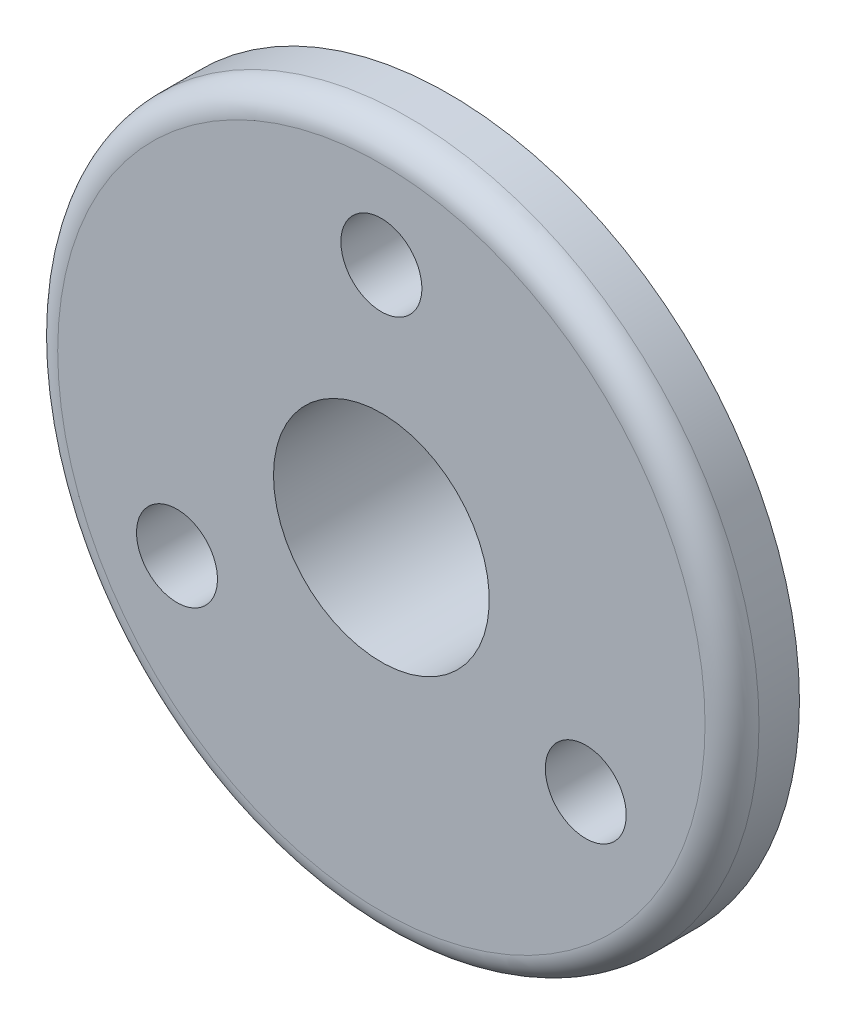
SolidWorks part; units mm, degrees
material "Plain Carbon Steel"
ref_plane "Front Plane" through (0, 0, 0) normal (0, 0, 1) x (1, 0, 0)
ref_plane "Top Plane" through (0, 0, 0) normal (0, 1, 0) x (1, 0, 0)
ref_plane "Right Plane" through (0, 0, 0) normal (1, 0, 0) x (0, 0, -1)
sketch "Flange Profile" plane through (0, 0, 0) normal (0, 0, 1) x (1, 0, 0)
  circle A0 centre (0, 0) radius 26
  dimension "D1" = 52
extrude "Flange Ø52" add sketch "Flange Profile" against normal blind 5
sketch "Hub Profile" plane through (0, 0, -5) normal (0, 0, -1) x (-1, 0, 0)
  circle A0 centre (0, 0) radius 12.5
  dimension "D1" = 25
extrude "Hub Ø25" add sketch "Hub Profile" along normal blind 7
sketch "Bore Profile" plane through (0, 0, -12) normal (0, 0, -1) x (-1, 0, 0)
  circle A0 centre (0, 0) radius 8
  dimension "D1" = 16
extrude "Bore Ø16" cut sketch "Bore Profile" against normal through all both
sketch "Bolt Hole Profile" plane through (0, 0, -5) normal (0, 0, -1) x (-1, 0, 0)
  line L0 (0, -28.5848) -> (0, 27.6798) construction
  line L1 (-29.4899, 0) -> (31.3754, 0) construction
  circle A0 centre (0, 17.5) radius 3
  circle A1 centre (0, 0) radius 17.5 construction
  circle A2 centre (15.1554, -8.75) radius 3
  circle A3 centre (-15.1554, -8.75) radius 3
  point P11 (0, 0)
  dimension "D1" = 6
  dimension "D2" = 35
  dimension "D3" = 3
extrude "Bolt Holes 3xØ6 PCD35" cut sketch "Bolt Hole Profile" against normal through all both
fillet "Flange Edge Fillet R2" radius 2 1 edges at (26, 0, 0)
